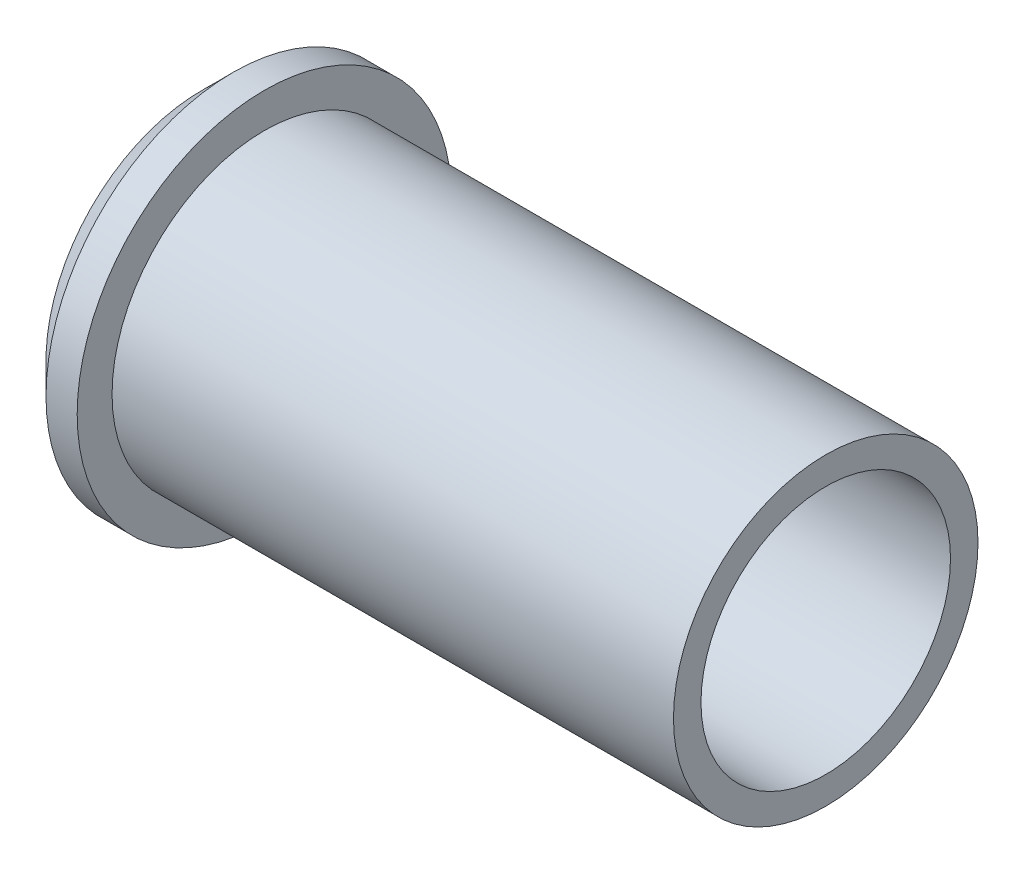
from build123d import *

# Parameters (mm, degrees)
EDGE_CHAMFER_0_0625IN_X_45DEG_SIZE = 1.5875


with BuildPart() as part:
    # Bushing Profile Sketch → Flanged Bushing Revolve (revolve)
    with BuildSketch(Plane.XY, mode=Mode.PRIVATE) as flanged_bushing_revolve_sk:
        Polygon((15.875, 6.35), (-15.875, 6.35), (-15.875, 8.89), (-15.875, 9.525), (-14.2875, 9.525), (-12.7, 9.525), (-12.7, 7.75), (15.875, 7.75), align=None)
    revolve(flanged_bushing_revolve_sk.sketch.rotate(Axis((40.781111111, 0, 0), (-1, 0, 0)), 90), axis=Axis((40.781111111, 0, 0), (-1, 0, 0)))

    # Edge Chamfer 0.0625in x 45deg
    edge_chamfer_0_0625in_x_45deg_edges = [part.edges().sort_by_distance(p)[0] for p in [
        (-15.875, 0, 9.525),
    ]]
    chamfer(edge_chamfer_0_0625in_x_45deg_edges, length=EDGE_CHAMFER_0_0625IN_X_45DEG_SIZE)


solid = part.part
